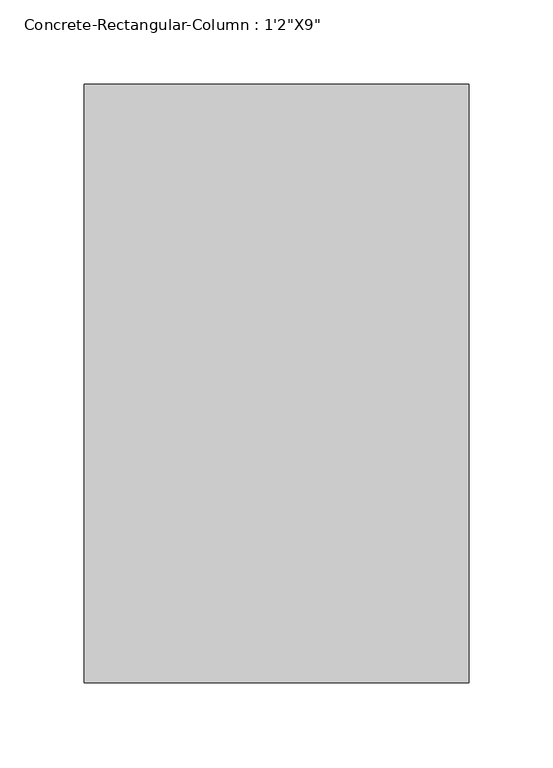
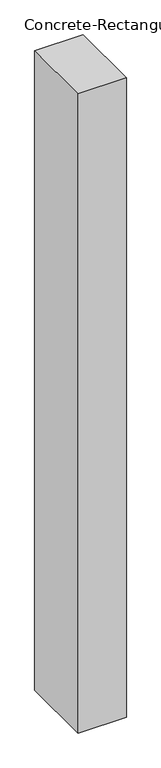
"""IFC4 building model written with IfcOpenShell, lengths in millimetres: column geometry."""

from ifc_helpers import new_model, si_unit, frame, origin, place, context, project, spatial, polyline, outline, extrude, source, transform, mapped, element, save


def column_2a2b4286(model_context):
    return source(origin(), model_context, "Body", "SweptSolid", [
        extrude(outline(polyline([(114.3, 177.8), (114.3, -177.8), (-114.3, -177.8), (-114.3, 177.8), (114.3, 177.8)])), frame((0.0, 0.0, 12801.6), z_axis=(0.0, 0.0, 1.0), x_axis=(1.0, 0.0, 0.0)), (0.0, 0.0, 1.0), 3200.4),
    ])


if __name__ == "__main__":
    model = new_model("IFC4")
    model_context = context("Model", 3, world=origin())
    ifc_project = project(units=[si_unit("LENGTHUNIT", "METRE", prefix="MILLI")], contexts=[model_context])
    site = spatial("IfcSite", under=ifc_project)
    building = spatial("IfcBuilding", under=site)
    placement = place(None, origin())
    column_shape = column_2a2b4286(model_context)
    element("IfcColumn", 1, ObjectType="Concrete-Rectangular-Column : 1'2\"X9\"", at=placement, inside=building, context=model_context, shape_type="MappedRepresentation", body=[
        mapped(column_shape, transform((0.0, 0.0, 0.0), x_axis=(1.0, 0.0, 0.0), y_axis=(0.0, 1.0, 0.0), z_axis=(0.0, 0.0, 1.0))),
    ])
    save(model, "model.ifc")

# Revit data of these elements
# Type "Concrete-Rectangular-Column : 1'2\"X9\""
#   Assembly Code = "B10"
#   b = 0' - 9"
#   h = 1' - 2"
#   Structural Material [instance default] = Concrete, Cast-in-Place gray
# Element 1 (IfcColumn, "Concrete-Rectangular-Column : 1'2\"X9\"")
#   Materials on its faces: "Concrete, Cast-in-Place gray"
# Materials
#   "Concrete, Cast-in-Place gray": class "Concrete", colour RGB 192 192 192, transparency 0, Description = "Cast-in-place concrete", Cost = 0
